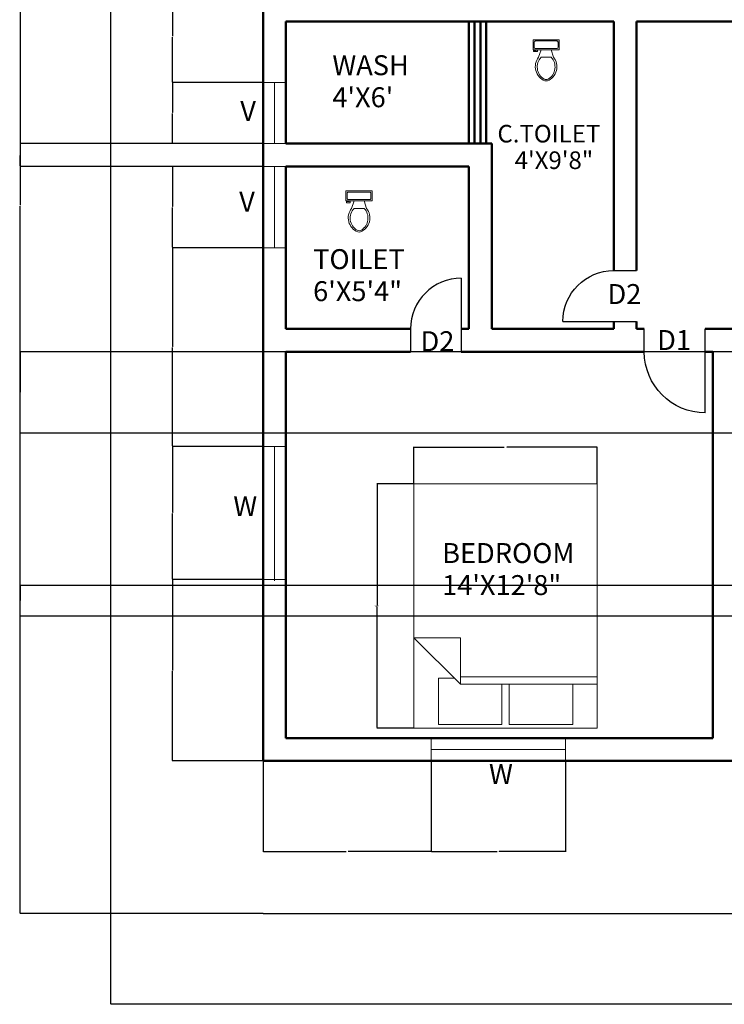
# Model space of a CAD drawing. Units: feet. Extents: x 1544 to 2324, y 1847 to 2475.
# Tile 1 of 4: x 1544 to 1821, y 1847 to 2234. Entities that reach past the tile are written whole.
import ezdxf

# ---------------------------------------------------------------- set-up
doc = ezdxf.new("R2010")
doc.units = ezdxf.units.FT
for name, color, linetype, lineweight in [('A-ANNO-DIMS', 2, 'Continuous', 18), ('A-ANNO-TEXT', 7, 'Continuous', 18), ('A-AREA-IDEN', 7, 'Continuous', 20), ('A-DOOR', 4, 'Continuous', 25), ('A-FLOR-FIXT', 9, 'Continuous', 18), ('A-FURN', 8, 'Continuous', 18), ('A-GLAZ', 4, 'Continuous', 18), ('A-WALL', 7, 'Continuous', 50), ('C-PROP', 3, 'Continuous', 25)]:
    doc.layers.add(name, color=color, linetype=linetype, lineweight=lineweight)
doc.styles.get("Standard").update_dxf_attribs({"font": 'arial.ttf'})
doc.dimstyles.get("Standard").update_dxf_attribs({"dimtxt": 0.18, "dimasz": 0.18, "dimexe": 0.18, "dimexo": 0.0625, "dimgap": 0.09, "dimtad": 0, "dimtih": 1, "dimtoh": 1, "dimdec": 4, "dimzin": 0, "dimdsep": 46, "dimtxsty": 'Standard', "dimcen": 0.09, "dimadec": 0, "dimazin": 0, "dimtfac": 1, "dimtdec": 4, "dimtofl": 0, "dimtmove": 0, "dimatfit": 3, "dimfxl": 1, "dimtolj": 1, "dimtzin": 0, "dimarcsym": 0})

# ---------------------------------------------------------------- blocks, each defined once
blk = doc.blocks.new('Bed - Queen')
for p, q in [((0, -80.00003), (0, 0)), ((0, 0), (59.99999, 0)), ((59.99999, 0), (59.99999, -80.00003)), ((7.99999, -1.2), (28.79998, -1.2)), ((7.99999, -14.4), (7.99999, -1.2)), ((28.79998, -1.2), (28.79998, -14.4)), ((31.19999, -1.2), (51.99999, -1.2)), ((31.19999, -14.4), (31.19999, -1.2)), ((51.99999, -1.2), (51.99999, -16.4)), ((0, -14.4), (44.8, -14.4)), ((59.99999, -29.6), (44.8, -14.4)), ((44.8, -14.4), (44.8, -29.6)), ((44.8, -16.8), (0, -16.8)), ((51.99999, -16.4), (46.79936, -16.4)), ((44.8, -29.6), (59.99999, -29.6)), ((59.99999, -80.00003), (0, -80.00003))]:
    blk.add_line(p, q)
blk = doc.blocks.new('Toilet - top')
for p, q in [((9.5, -6), (9.5, -2)), ((-10, -8.5), (-8, -8.5)), ((-10, -9.5), (-10, -8.5)), ((-7, -9.5), (-10, -9.5)), ((-8, -8.5), (-8, -8)), ((-7, -8), (-7, -9.5)), ((-4, -8), (-6, -14)), ((4, -14), (-4, -14)), ((4, -8), (6, -14))]:
    blk.add_line(p, q)
blk.add_lwpolyline([(10.5, -8), (10.5, 0), (-10.5, 0), (-10.5, -8)], close=True)
for points in [[(-9.5, -2), (-9.5, -6)], [(8.5, -1), (-8.5, -1)], [(-8.5, -7), (8.5, -7)]]:
    blk.add_lwpolyline(points)
for centre, radius, start, end in [((-8.62, -1.88), 0.884, 81.8699, 188.1301), ((-8.62, -6.12), 0.884, 171.8699, 278.1301), ((8.62, -1.88), 0.884, 351.8699, 98.1301), ((8.62, -6.12), 0.884, 261.8699, 8.1301), ((3.52, -21.58), 12.17, 141.46911, 247.97143), ((4.2, -21.82), 11.33, 136.36773, 238.94682), ((-3.52, -21.58), 12.17, 292.02843, 38.53071), ((-4.2, -21.82), 11.33, 301.05301, 43.63209), ((0, -27.88), 4, 245.73182, 294.26817), ((0, -29), 4, 254.86053, 285.13947)]:
    blk.add_arc(centre, radius, start, end)
blk = doc.blocks.new('DOOR-SINGLE-R24')
for p, q in [((9, 24), (0, 24)), ((33, 0), (0, 0))]:
    blk.add_line(p, q)
blk.add_arc((9, 0), 24, 0, 90)
blk = doc.blocks.new('DOOR-SINGLE-R20')
for p, q in [((20, 29), (20, 0)), ((0, 9), (0, 0))]:
    blk.add_line(p, q)
blk.add_arc((20, 9), 20, 90, 180)
blk = doc.blocks.new('*D17')
at = {"layer": 'A-ANNO-DIMS', "color": 0, "lineweight": -2, "transparency": 16777216}
for p, q in [((1698.86, 2051.73), (1684.32, 2051.73)), ((1684.5, 2051.55), (1684.5, 2003.85)), ((1684.5, 1955.77), (1684.5, 2003.47)), ((1698.86, 1955.59), (1684.32, 1955.59))]:
    blk.add_line(p, q, dxfattribs=at)
at = {"layer": 'A-ANNO-DIMS', "color": 0, "transparency": 16777216}
for points in [[(1684.47, 2051.55), (1684.53, 2051.55), (1684.5, 2051.73)], [(1684.47, 1955.77), (1684.53, 1955.77), (1684.5, 1955.59)]]:
    blk.add_solid(points, dxfattribs=at)
at = {"layer": 'Defpoints', "color": 0, "transparency": 16777216}
for p in [(1698.93, 2051.73), (1684.5, 1955.59), (1698.93, 1955.59)]:
    blk.add_point(p, dxfattribs=at)
at = {"layer": 'A-ANNO-DIMS', "color": 0, "transparency": 16777216, "insert": (1684.5, 2003.66), "char_height": 0.18, "attachment_point": 5}
blk.add_mtext('\\A1;QUEEN BED 96 TYP.', dxfattribs=at)
blk = doc.blocks.new('*D18')
at = {"layer": 'A-ANNO-DIMS', "color": 0, "lineweight": -2, "transparency": 16777216}
for p, q in [((1698.93, 2051.8), (1698.93, 2066.34)), ((1699.11, 2066.16), (1734.45, 2066.16)), ((1770.85, 2066.16), (1735.51, 2066.16)), ((1771.03, 2051.8), (1771.03, 2066.34))]:
    blk.add_line(p, q, dxfattribs=at)
at = {"layer": 'A-ANNO-DIMS', "color": 0, "transparency": 16777216}
for points in [[(1699.11, 2066.19), (1699.11, 2066.13), (1698.93, 2066.16)], [(1770.85, 2066.19), (1770.85, 2066.13), (1771.03, 2066.16)]]:
    blk.add_solid(points, dxfattribs=at)
at = {"layer": 'Defpoints', "color": 0, "transparency": 16777216}
for p in [(1698.93, 2066.16), (1698.93, 2051.73), (1771.03, 2051.73)]:
    blk.add_point(p, dxfattribs=at)
at = {"layer": 'A-ANNO-DIMS', "color": 0, "transparency": 16777216, "insert": (1734.98, 2066.16), "char_height": 0.18, "attachment_point": 5}
blk.add_mtext('\\A1;72 TYP.', dxfattribs=at)
blk = doc.blocks.new('*D31')
at = {"layer": 'A-ANNO-DIMS', "color": 0, "lineweight": -2, "transparency": 16777216}
for p, q in [((1579.55, 1882.61), (1579.55, 1846.89)), ((2288.55, 1882.61), (2288.55, 1846.89)), ((1579.73, 1847.07), (1933.77, 1847.07)), ((2288.37, 1847.07), (1934.34, 1847.07))]:
    blk.add_line(p, q, dxfattribs=at)
at = {"layer": 'A-ANNO-DIMS', "color": 0, "transparency": 16777216}
for points in [[(1579.73, 1847.1), (1579.73, 1847.04), (1579.55, 1847.07)], [(2288.37, 1847.1), (2288.37, 1847.04), (2288.55, 1847.07)]]:
    blk.add_solid(points, dxfattribs=at)
at = {"layer": 'Defpoints', "color": 0, "transparency": 16777216}
for p in [(1579.55, 1882.67), (2288.55, 1882.67), (2288.55, 1847.07)]:
    blk.add_point(p, dxfattribs=at)
at = {"layer": 'A-ANNO-DIMS', "color": 0, "transparency": 16777216, "insert": (1934.05, 1847.07), "char_height": 0.18, "attachment_point": 5}
blk.add_mtext('\\A1;709', dxfattribs=at)
blk = doc.blocks.new('*D32')
at = {"layer": 'A-ANNO-DIMS', "color": 0, "lineweight": -2, "transparency": 16777216}
for p, q in [((1579.49, 2439.67), (1543.77, 2439.67)), ((1543.95, 2439.49), (1543.95, 2161.35)), ((1543.95, 1882.85), (1543.95, 2160.99)), ((1579.49, 1882.67), (1543.77, 1882.67))]:
    blk.add_line(p, q, dxfattribs=at)
at = {"layer": 'A-ANNO-DIMS', "color": 0, "transparency": 16777216}
for points in [[(1543.92, 2439.49), (1543.98, 2439.49), (1543.95, 2439.67)], [(1543.92, 1882.85), (1543.98, 1882.85), (1543.95, 1882.67)]]:
    blk.add_solid(points, dxfattribs=at)
at = {"layer": 'Defpoints', "color": 0, "transparency": 16777216}
for p in [(1543.95, 2439.67), (1579.55, 2439.67), (1579.55, 1882.67)]:
    blk.add_point(p, dxfattribs=at)
at = {"layer": 'A-ANNO-DIMS', "color": 0, "transparency": 16777216, "insert": (1543.95, 2161.17), "char_height": 0.18, "attachment_point": 5}
blk.add_mtext('\\A1;557', dxfattribs=at)
blk = doc.blocks.new('*D54')
at = {"layer": 'A-ANNO-DIMS', "color": 0, "lineweight": -2, "transparency": 16777216}
for p, q in [((1825.49, 2011.67), (1543.77, 2011.67)), ((1543.95, 2011.49), (1543.95, 2005.85)), ((1543.95, 1999.85), (1543.95, 2005.49)), ((1825.49, 1999.67), (1543.77, 1999.67))]:
    blk.add_line(p, q, dxfattribs=at)
at = {"layer": 'A-ANNO-DIMS', "color": 0, "transparency": 16777216}
for points in [[(1543.92, 2011.49), (1543.98, 2011.49), (1543.95, 2011.67)], [(1543.92, 1999.85), (1543.98, 1999.85), (1543.95, 1999.67)]]:
    blk.add_solid(points, dxfattribs=at)
at = {"layer": 'Defpoints', "color": 0, "transparency": 16777216}
for p in [(1825.55, 2011.67), (1543.95, 1999.67), (1825.55, 1999.67)]:
    blk.add_point(p, dxfattribs=at)
at = {"layer": 'A-ANNO-DIMS', "color": 0, "transparency": 16777216, "insert": (1543.95, 2005.67), "char_height": 0.18, "attachment_point": 5}
blk.add_mtext('\\A1;12', dxfattribs=at)
blk = doc.blocks.new('*D55')
at = {"layer": 'A-ANNO-DIMS', "color": 0, "lineweight": -2, "transparency": 16777216}
for p, q in [((1921.49, 2103.67), (1543.77, 2103.67)), ((1543.95, 2103.49), (1543.95, 2087.85)), ((1543.95, 2071.85), (1543.95, 2087.49)), ((1921.49, 2071.67), (1543.77, 2071.67))]:
    blk.add_line(p, q, dxfattribs=at)
at = {"layer": 'A-ANNO-DIMS', "color": 0, "transparency": 16777216}
for points in [[(1543.92, 2103.49), (1543.98, 2103.49), (1543.95, 2103.67)], [(1543.92, 2071.85), (1543.98, 2071.85), (1543.95, 2071.67)]]:
    blk.add_solid(points, dxfattribs=at)
at = {"layer": 'Defpoints', "color": 0, "transparency": 16777216}
for p in [(1543.95, 2103.67), (1921.55, 2103.67), (1921.55, 2071.67)]:
    blk.add_point(p, dxfattribs=at)
at = {"layer": 'A-ANNO-DIMS', "color": 0, "transparency": 16777216, "insert": (1543.95, 2087.67), "char_height": 0.18, "attachment_point": 5}
blk.add_mtext('\\A1;32', dxfattribs=at)
blk = doc.blocks.new('*D57')
at = {"layer": 'A-ANNO-DIMS', "color": 0, "lineweight": -2, "transparency": 16777216}
for p, q in [((1639.49, 2014.02), (1603.77, 2014.02)), ((1603.95, 2013.84), (1603.95, 1978.53)), ((1603.95, 1942.85), (1603.95, 1978.16)), ((1639.49, 1942.67), (1603.77, 1942.67))]:
    blk.add_line(p, q, dxfattribs=at)
at = {"layer": 'A-ANNO-DIMS', "color": 0, "transparency": 16777216}
for points in [[(1603.92, 2013.84), (1603.98, 2013.84), (1603.95, 2014.02)], [(1603.92, 1942.85), (1603.98, 1942.85), (1603.95, 1942.67)]]:
    blk.add_solid(points, dxfattribs=at)
at = {"layer": 'Defpoints', "color": 0, "transparency": 16777216}
for p in [(1603.95, 2014.02), (1639.55, 2014.02), (1639.55, 1942.67)]:
    blk.add_point(p, dxfattribs=at)
at = {"layer": 'A-ANNO-DIMS', "color": 0, "transparency": 16777216, "insert": (1603.95, 1978.34), "char_height": 0.18, "attachment_point": 5}
blk.add_mtext('\\A1;71.35', dxfattribs=at)
blk = doc.blocks.new('*D58')
at = {"layer": 'A-ANNO-DIMS', "color": 0, "lineweight": -2, "transparency": 16777216}
for p, q in [((1639.49, 2066.47), (1603.77, 2066.47)), ((1603.95, 2066.29), (1603.95, 2040.42)), ((1603.95, 2014.2), (1603.95, 2040.06)), ((1639.49, 2014.02), (1603.77, 2014.02))]:
    blk.add_line(p, q, dxfattribs=at)
at = {"layer": 'A-ANNO-DIMS', "color": 0, "transparency": 16777216}
for points in [[(1603.92, 2066.29), (1603.98, 2066.29), (1603.95, 2066.47)], [(1603.92, 2014.2), (1603.98, 2014.2), (1603.95, 2014.02)]]:
    blk.add_solid(points, dxfattribs=at)
at = {"layer": 'Defpoints', "color": 0, "transparency": 16777216}
for p in [(1603.95, 2066.47), (1639.55, 2066.47), (1639.55, 2014.02)]:
    blk.add_point(p, dxfattribs=at)
at = {"layer": 'A-ANNO-DIMS', "color": 0, "transparency": 16777216, "insert": (1603.95, 2040.24), "char_height": 0.18, "attachment_point": 5}
blk.add_mtext('\\A1;52.45', dxfattribs=at)
blk = doc.blocks.new('*D59')
at = {"layer": 'A-ANNO-DIMS', "color": 0, "lineweight": -2, "transparency": 16777216}
for p, q in [((1639.49, 2144.67), (1603.77, 2144.67)), ((1603.95, 2144.49), (1603.95, 2105.75)), ((1603.95, 2066.65), (1603.95, 2105.39)), ((1639.49, 2066.47), (1603.77, 2066.47))]:
    blk.add_line(p, q, dxfattribs=at)
at = {"layer": 'A-ANNO-DIMS', "color": 0, "transparency": 16777216}
for points in [[(1603.92, 2144.49), (1603.98, 2144.49), (1603.95, 2144.67)], [(1603.92, 2066.65), (1603.98, 2066.65), (1603.95, 2066.47)]]:
    blk.add_solid(points, dxfattribs=at)
at = {"layer": 'Defpoints', "color": 0, "transparency": 16777216}
for p in [(1603.95, 2144.67), (1639.55, 2144.67), (1639.55, 2066.47)]:
    blk.add_point(p, dxfattribs=at)
at = {"layer": 'A-ANNO-DIMS', "color": 0, "transparency": 16777216, "insert": (1603.95, 2105.57), "char_height": 0.18, "attachment_point": 5}
blk.add_mtext('\\A1;78.2', dxfattribs=at)
blk = doc.blocks.new('*D60')
at = {"layer": 'A-ANNO-DIMS', "color": 0, "lineweight": -2, "transparency": 16777216}
for p, q in [((1639.49, 2176.67), (1603.77, 2176.67)), ((1603.95, 2176.49), (1603.95, 2160.85)), ((1603.95, 2144.85), (1603.95, 2160.49)), ((1639.49, 2144.67), (1603.77, 2144.67))]:
    blk.add_line(p, q, dxfattribs=at)
at = {"layer": 'A-ANNO-DIMS', "color": 0, "transparency": 16777216}
for points in [[(1603.92, 2176.49), (1603.98, 2176.49), (1603.95, 2176.67)], [(1603.92, 2144.85), (1603.98, 2144.85), (1603.95, 2144.67)]]:
    blk.add_solid(points, dxfattribs=at)
at = {"layer": 'Defpoints', "color": 0, "transparency": 16777216}
for p in [(1603.95, 2176.67), (1639.55, 2176.67), (1639.55, 2144.67)]:
    blk.add_point(p, dxfattribs=at)
at = {"layer": 'A-ANNO-DIMS', "color": 0, "transparency": 16777216, "insert": (1603.95, 2160.67), "char_height": 0.18, "attachment_point": 5}
blk.add_mtext('\\A1;32', dxfattribs=at)
blk = doc.blocks.new('*D61')
at = {"layer": 'A-ANNO-DIMS', "color": 0, "lineweight": -2, "transparency": 16777216}
for p, q in [((1639.49, 2185.67), (1543.77, 2185.67)), ((1543.95, 2185.49), (1543.95, 2181.35)), ((1543.95, 2176.85), (1543.95, 2180.99)), ((1639.49, 2176.67), (1543.77, 2176.67))]:
    blk.add_line(p, q, dxfattribs=at)
at = {"layer": 'A-ANNO-DIMS', "color": 0, "transparency": 16777216}
for points in [[(1543.92, 2185.49), (1543.98, 2185.49), (1543.95, 2185.67)], [(1543.92, 2176.85), (1543.98, 2176.85), (1543.95, 2176.67)]]:
    blk.add_solid(points, dxfattribs=at)
at = {"layer": 'Defpoints', "color": 0, "transparency": 16777216}
for p in [(1543.95, 2185.67), (1639.55, 2185.67), (1639.55, 2176.67)]:
    blk.add_point(p, dxfattribs=at)
at = {"layer": 'A-ANNO-DIMS', "color": 0, "transparency": 16777216, "insert": (1543.95, 2181.17), "char_height": 0.18, "attachment_point": 5}
blk.add_mtext('\\A1;9', dxfattribs=at)
blk = doc.blocks.new('*D62')
at = {"layer": 'A-ANNO-DIMS', "color": 0, "lineweight": -2, "transparency": 16777216}
for p, q in [((1639.49, 2209.67), (1603.77, 2209.67)), ((1603.95, 2209.49), (1603.95, 2197.85)), ((1603.95, 2185.85), (1603.95, 2197.49)), ((1639.49, 2185.67), (1603.77, 2185.67))]:
    blk.add_line(p, q, dxfattribs=at)
at = {"layer": 'A-ANNO-DIMS', "color": 0, "transparency": 16777216}
for points in [[(1603.92, 2209.49), (1603.98, 2209.49), (1603.95, 2209.67)], [(1603.92, 2185.85), (1603.98, 2185.85), (1603.95, 2185.67)]]:
    blk.add_solid(points, dxfattribs=at)
at = {"layer": 'Defpoints', "color": 0, "transparency": 16777216}
for p in [(1603.95, 2209.67), (1639.55, 2209.67), (1639.55, 2185.67)]:
    blk.add_point(p, dxfattribs=at)
at = {"layer": 'A-ANNO-DIMS', "color": 0, "transparency": 16777216, "insert": (1603.95, 2197.67), "char_height": 0.18, "attachment_point": 5}
blk.add_mtext('\\A1;24', dxfattribs=at)
blk = doc.blocks.new('*D63')
at = {"layer": 'A-ANNO-DIMS', "color": 0, "lineweight": -2, "transparency": 16777216}
for p, q in [((1639.49, 2245.67), (1603.77, 2245.67)), ((1603.95, 2245.49), (1603.95, 2227.85)), ((1603.95, 2209.85), (1603.95, 2227.49)), ((1639.49, 2209.67), (1603.77, 2209.67))]:
    blk.add_line(p, q, dxfattribs=at)
at = {"layer": 'A-ANNO-DIMS', "color": 0, "transparency": 16777216}
for points in [[(1603.92, 2245.49), (1603.98, 2245.49), (1603.95, 2245.67)], [(1603.92, 2209.85), (1603.98, 2209.85), (1603.95, 2209.67)]]:
    blk.add_solid(points, dxfattribs=at)
at = {"layer": 'Defpoints', "color": 0, "transparency": 16777216}
for p in [(1603.95, 2245.67), (1639.55, 2245.67), (1639.55, 2209.67)]:
    blk.add_point(p, dxfattribs=at)
at = {"layer": 'A-ANNO-DIMS', "color": 0, "transparency": 16777216, "insert": (1603.95, 2227.67), "char_height": 0.18, "attachment_point": 5}
blk.add_mtext('\\A1;36', dxfattribs=at)
blk = doc.blocks.new('*D66')
at = {"layer": 'A-ANNO-DIMS', "color": 0, "lineweight": -2, "transparency": 16777216}
for p, q in [((1639.55, 1942.61), (1639.55, 1906.89)), ((1705.67, 1942.61), (1705.67, 1906.89)), ((1639.73, 1907.07), (1672.23, 1907.07)), ((1705.49, 1907.07), (1672.99, 1907.07))]:
    blk.add_line(p, q, dxfattribs=at)
at = {"layer": 'A-ANNO-DIMS', "color": 0, "transparency": 16777216}
for points in [[(1639.73, 1907.1), (1639.73, 1907.04), (1639.55, 1907.07)], [(1705.49, 1907.1), (1705.49, 1907.04), (1705.67, 1907.07)]]:
    blk.add_solid(points, dxfattribs=at)
at = {"layer": 'Defpoints', "color": 0, "transparency": 16777216}
for p in [(1639.55, 1942.67), (1705.67, 1942.67), (1639.55, 1907.07)]:
    blk.add_point(p, dxfattribs=at)
at = {"layer": 'A-ANNO-DIMS', "color": 0, "transparency": 16777216, "insert": (1672.61, 1907.07), "char_height": 0.18, "attachment_point": 5}
blk.add_mtext('\\A1;66.11', dxfattribs=at)
blk = doc.blocks.new('*D67')
at = {"layer": 'A-ANNO-DIMS', "color": 0, "lineweight": -2, "transparency": 16777216}
for p, q in [((1705.67, 1942.61), (1705.67, 1906.89)), ((1758.52, 1942.61), (1758.52, 1906.89)), ((1705.85, 1907.07), (1731.7, 1907.07)), ((1758.34, 1907.07), (1732.49, 1907.07))]:
    blk.add_line(p, q, dxfattribs=at)
at = {"layer": 'A-ANNO-DIMS', "color": 0, "transparency": 16777216}
for points in [[(1705.85, 1907.1), (1705.85, 1907.04), (1705.67, 1907.07)], [(1758.34, 1907.1), (1758.34, 1907.04), (1758.52, 1907.07)]]:
    blk.add_solid(points, dxfattribs=at)
at = {"layer": 'Defpoints', "color": 0, "transparency": 16777216}
for p in [(1705.67, 1942.67), (1758.52, 1942.67), (1705.67, 1907.07)]:
    blk.add_point(p, dxfattribs=at)
at = {"layer": 'A-ANNO-DIMS', "color": 0, "transparency": 16777216, "insert": (1732.09, 1907.07), "char_height": 0.18, "attachment_point": 5}
blk.add_mtext('\\A1;52.85', dxfattribs=at)

msp = doc.modelspace()

# ---------------------------------------------------------------- linework, layer by layer
at = {"layer": 'A-GLAZ'}
for p, q in [((1648.5539, 2209.6692), (1639.5539, 2209.6692)), ((1644.0539, 2209.6692), (1644.0539, 2185.6692)), ((1648.5539, 2185.6692), (1639.5539, 2185.6692)), ((1648.5539, 2176.6692), (1639.5539, 2176.6692)), ((1644.0539, 2144.6692), (1644.0539, 2176.6692)), ((1648.5539, 2144.6692), (1639.5539, 2144.6692)), ((1648.5539, 2066.4654), (1639.5539, 2066.4654)), ((1644.0539, 2066.4654), (1644.0539, 2013.5998)), ((1639.5539, 2014.017), (1648.5539, 2014.017)), ((1705.6665, 1951.6692), (1705.6665, 1942.6692)), ((1758.5209, 1951.6692), (1758.5209, 1942.6692)), ((1705.6665, 1947.1692), (1758.5209, 1947.1692))]:
    msp.add_line(p, q, dxfattribs=at)
at = {"layer": 'A-WALL'}
for p, q in [((1639.5539, 1942.6692), (1639.5539, 2245.6692)), ((1639.5539, 2233.6692), (1639.5539, 1942.6692)), ((1648.5539, 2233.6692), (1648.5539, 2185.6692)), ((1729.5539, 2233.6692), (1648.5539, 2233.6692)), ((1720.5539, 2185.6692), (1720.5539, 2233.6692)), ((1722.8039, 2185.6692), (1722.8039, 2233.6692)), ((1725.0539, 2185.6692), (1725.0539, 2233.6692)), ((1727.3039, 2185.6692), (1727.3039, 2233.6692)), ((1777.5539, 2233.6692), (1729.5539, 2233.6692)), ((1777.5539, 2135.6692), (1777.5539, 2233.6692)), ((1913.5539, 2233.6692), (1786.5539, 2233.6692)), ((1786.5539, 2135.6692), (1786.5539, 2233.6692)), ((1648.5539, 2185.6692), (1729.5539, 2185.6692)), ((1729.5539, 2112.6692), (1729.5539, 2185.6692)), ((1639.5539, 2176.6692), (1639.5539, 2112.6692)), ((1648.5539, 2176.6692), (1720.5539, 2176.6692)), ((1648.5539, 2176.6692), (1648.5539, 2112.6692)), ((1720.5539, 2112.6692), (1720.5539, 2176.6692)), ((1648.5539, 2112.6692), (1697.5539, 2112.6692)), ((1717.5539, 2112.6692), (1720.5539, 2112.6692)), ((1729.5539, 2112.6692), (1777.5539, 2112.6692)), ((1777.5539, 2112.6692), (1729.5539, 2112.6692)), ((1777.5539, 2112.6692), (1777.5539, 2115.6692)), ((1786.5539, 2112.6692), (1786.5539, 2115.6692)), ((1786.5539, 2112.6692), (1789.5539, 2112.6692)), ((1789.5539, 2112.6692), (1786.5539, 2112.6692)), ((1816.5539, 2112.6692), (1813.5539, 2112.6692)), ((1813.5539, 2112.6692), (1828.5539, 2112.6692)), ((1639.5539, 2103.6692), (1639.5539, 1942.6692)), ((1648.5539, 2103.6692), (1697.5539, 2103.6692)), ((1648.5539, 2103.6692), (1648.5539, 1951.6692)), ((1717.5539, 2103.6692), (1720.5539, 2103.6692)), ((1789.5539, 2103.6692), (1720.5539, 2103.6692)), ((1816.5539, 2103.6692), (1813.5539, 2103.6692)), ((1816.5539, 1951.6692), (1816.5539, 2103.6692)), ((1648.5539, 1951.6692), (1816.5539, 1951.6692)), ((1639.5539, 1942.6692), (1816.5539, 1942.6692)), ((1639.5539, 1942.6692), (1921.5539, 1942.6692)), ((1639.5539, 1942.6692), (2031.5539, 1942.6692))]:
    msp.add_line(p, q, dxfattribs=at)
at = {"layer": 'C-PROP'}
for p, q in [((1579.5539, 1882.6692), (1579.5539, 2439.6692)), ((1639.5539, 1882.6692), (1579.5539, 1882.6692)), ((1639.5539, 1882.6692), (2288.5539, 1882.6692))]:
    msp.add_line(p, q, dxfattribs=at)

# ---------------------------------------------------------------- block references
at = {"layer": 'A-DOOR', "extrusion": (0, 0, -1), "zscale": -1}
for name, p, rotation in [('DOOR-SINGLE-R20', (-1786.5541, 2135.6691), 270.0000000000006), ('DOOR-SINGLE-R24', (-1813.5541, 2112.6691), 270)]:
    msp.add_blockref(name, p, dxfattribs=dict(at, rotation=rotation))
at = {"layer": 'A-DOOR'}
msp.add_blockref('DOOR-SINGLE-R20', (1697.554, 2103.669), dxfattribs=at)
at = {"layer": 'A-FLOR-FIXT', "xscale": 0.4921201164889298, "yscale": 0.4921201164889298, "zscale": 0.4921201164889298}
for p in [(1750.9327, 2226.5154), (1677.3162, 2167.0434)]:
    msp.add_blockref('Toilet - top', p, dxfattribs=at)
at = {"layer": 'A-FURN', "xscale": 1.20179462178574, "yscale": 1.20179462178574, "zscale": 1.20179462178574, "rotation": 180}
msp.add_blockref('Bed - Queen', (1771.0339, 1955.5909), dxfattribs=at)

# ---------------------------------------------------------------- texts
at = {"layer": 'A-ANNO-TEXT'}
for s, height, p in [('V', 7.8492, (1630.5562, 2194.5342)), ('V', 7.8492, (1630.1343, 2158.8464)), ('D2', 7.84917, (1775.0903, 2122.4953)), ('D2', 7.84917, (1701.5031, 2103.9411)), ('D1', 7.84917, (1794.6264, 2104.3982)), ('W', 7.8492, (1627.8159, 2039.0211)), ('W', 7.8492, (1728.4417, 1933.5922))]:
    msp.add_text(s, height=height, dxfattribs=at).set_placement(p)
at = {"layer": 'A-AREA-IDEN'}
for s, height, p in [('WASH', 7.84917, (1666.7971, 2212.557)), ("4'X6'", 7.84917, (1666.7971, 2199.948)), ('C.TOILET', 6.93413, (1731.7644, 2186.0716)), ('4\'X9\'8"', 6.93413, (1738.5452, 2175.6269)), ('TOILET', 7.84917, (1659.2361, 2136.2354)), ('6\'X5\'4"', 7.84917, (1659.2361, 2123.6264)), ('BEDROOM', 7.84917, (1710.0125, 2020.5626)), ('14\'X12\'8"', 7.84917, (1710.0125, 2007.9536))]:
    msp.add_text(s, height=height, dxfattribs=at).set_placement(p)

# ---------------------------------------------------------------- dimensions: what is measured, and where the dimension line sits
at = {"layer": 'A-ANNO-DIMS'}
for base, p1, p2, angle, override, picture, middle in [((1543.9539, 2439.6692), (1579.5539, 1882.6692), (1579.5539, 2439.6692), 90, {"dimdec": 0, "dimlfac": 1, "dimrnd": 0, "dimzin": 0, "dimdsep": 46, "dimlunit": 2}, '*D32', (1543.9539, 2161.1692)), ((1603.9539, 2245.6692), (1639.5539, 2209.6692), (1639.5539, 2245.6692), 90, {"dimdec": 0, "dimlfac": 1, "dimrnd": 0, "dimzin": 0, "dimdsep": 46, "dimlunit": 2}, '*D63', (1603.9539, 2227.6692)), ((1603.9539, 2209.6692), (1639.5539, 2185.6692), (1639.5539, 2209.6692), 90, {"dimdec": 0, "dimlfac": 1, "dimrnd": 0, "dimzin": 0, "dimdsep": 46, "dimlunit": 2}, '*D62', (1603.9539, 2197.6692)), ((1543.9539, 2185.6692), (1639.5539, 2176.6692), (1639.5539, 2185.6692), 90, {"dimdec": 0, "dimlfac": 1, "dimrnd": 0, "dimzin": 0, "dimdsep": 46, "dimlunit": 2}, '*D61', (1543.9539, 2181.1692)), ((1603.9539, 2176.6692), (1639.5539, 2144.6692), (1639.5539, 2176.6692), 90, {"dimdec": 0, "dimlfac": 1, "dimrnd": 0, "dimzin": 0, "dimdsep": 46, "dimlunit": 2}, '*D60', (1603.9539, 2160.6692)), ((1603.9539, 2144.6692), (1639.5539, 2066.4654), (1639.5539, 2144.6692), 90, {"dimdec": 1, "dimlfac": 1, "dimrnd": 0, "dimzin": 0, "dimdsep": 46, "dimlunit": 2}, '*D59', (1603.9539, 2105.5673)), ((1543.9539, 2103.6692), (1921.5539, 2071.6692), (1921.5539, 2103.6692), 90, {"dimdec": 0, "dimlfac": 1, "dimrnd": 0, "dimzin": 0, "dimdsep": 46, "dimlunit": 2}, '*D55', (1543.9539, 2087.6692)), ((1603.9539, 2066.4654), (1639.5539, 2014.017), (1639.5539, 2066.4654), 90, {"dimdec": 2, "dimlfac": 1, "dimrnd": 0, "dimzin": 0, "dimdsep": 46, "dimlunit": 2}, '*D58', (1603.9539, 2040.2412)), ((1543.9539, 1999.6692), (1825.5539, 2011.6692), (1825.5539, 1999.6692), 90, {"dimdec": 0, "dimlfac": 1, "dimrnd": 0, "dimzin": 0, "dimdsep": 46, "dimlunit": 2}, '*D54', (1543.9539, 2005.6692)), ((1603.9539, 2014.017), (1639.5539, 1942.6692), (1639.5539, 2014.017), 90, {"dimdec": 2, "dimlfac": 1, "dimrnd": 0, "dimzin": 0, "dimdsep": 46, "dimlunit": 2}, '*D57', (1603.9539, 1978.3431)), ((1639.5539, 1907.0692), (1705.6665, 1942.6692), (1639.5539, 1942.6692), 180, {"dimdec": 2, "dimlfac": 1, "dimrnd": 0, "dimzin": 0, "dimdsep": 46, "dimlunit": 2}, '*D66', (1672.6102, 1907.0692)), ((1705.6665, 1907.0692), (1758.5209, 1942.6692), (1705.6665, 1942.6692), 180, {"dimdec": 2, "dimlfac": 1, "dimrnd": 0, "dimzin": 0, "dimdsep": 46, "dimlunit": 2}, '*D67', (1732.0937, 1907.0692))]:
    dim = msp.add_linear_dim(base=base, p1=p1, p2=p2, angle=angle, dimstyle='Standard', override=override, dxfattribs=at)
    dim.commit()
    dim.dimension.update_dxf_attribs({"geometry": picture, "text_midpoint": middle})
for base, p1, p2, angle, text, picture, middle in [((1698.9263, 2066.1561), (1771.0339, 2051.7345), (1698.9263, 2051.7345), 180, '<> TYP.', '*D18', (1734.9801, 2066.1561)), ((1684.5047, 1955.5909), (1698.9263, 2051.7345), (1698.9263, 1955.5909), 270, 'QUEEN BED <> TYP.', '*D17', (1684.5047, 2003.6627))]:
    dim = msp.add_linear_dim(base=base, p1=p1, p2=p2, angle=angle, text=text, dimstyle='Standard', override={"dimdec": 0, "dimlfac": 1, "dimrnd": 0, "dimzin": 0, "dimdsep": 46, "dimlunit": 2}, dxfattribs=at)
    dim.commit()
    dim.dimension.update_dxf_attribs({"geometry": picture, "text_midpoint": middle})
dim = msp.add_linear_dim(base=(2288.5539, 1847.0692), p1=(1579.5539, 1882.6692), p2=(2288.5539, 1882.6692), dimstyle='Standard', override={"dimdec": 0, "dimlfac": 1, "dimrnd": 0, "dimzin": 0, "dimdsep": 46, "dimlunit": 2}, dxfattribs=at)
dim.commit()
dim.dimension.update_dxf_attribs({"geometry": '*D31', "text_midpoint": (1934.0539, 1847.0692)})

doc.saveas('drawing.dxf')
